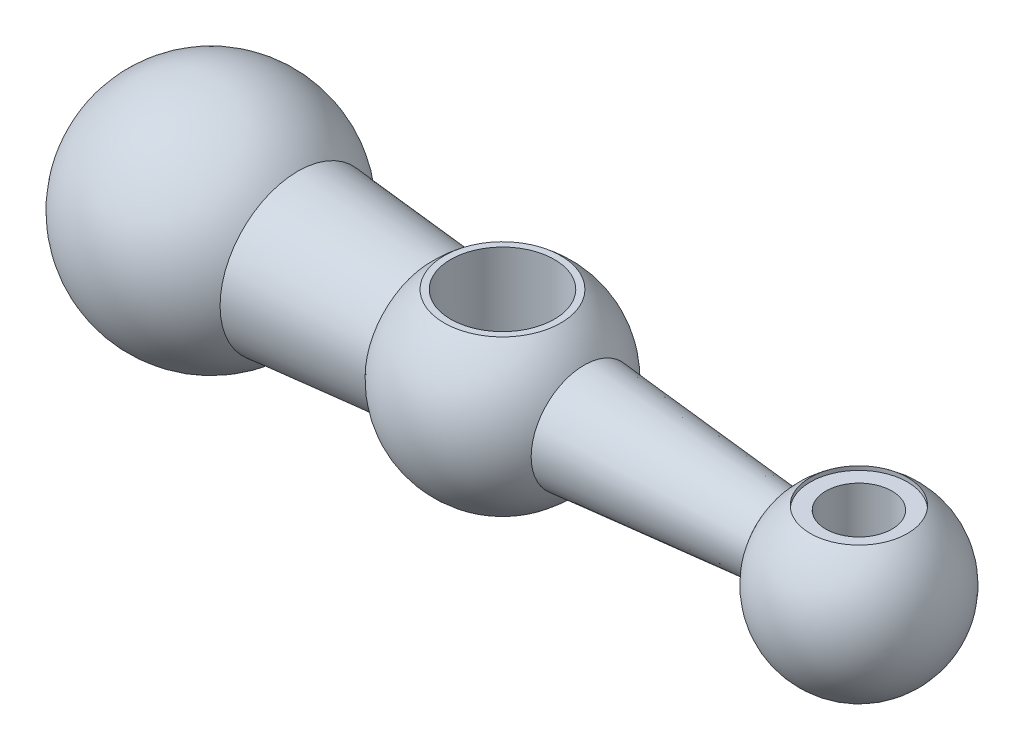
SolidWorks part; units mm, degrees
material "Plain Carbon Steel"
ref_plane "Front Plane" through (0, 0, 0) normal (0, 0, 1) x (1, 0, 0)
ref_plane "Top Plane" through (0, 0, 0) normal (0, 1, 0) x (1, 0, 0)
ref_plane "Right Plane" through (0, 0, 0) normal (1, 0, 0) x (0, 0, -1)
sketch "Handle Profile Sketch" plane through (0, 0, 0) normal (0, 0, 1) x (1, 0, 0)
  line L0 (-65.4913, 0) -> (73.3358, 0) construction
  line L1 (-31.5836, 12) -> (-10.9885, 10.2104)
  line L2 (-63, 0) -> (68, 0)
  line L3 (12.5849, 8.162) -> (43.2208, 5.5)
  arc A0 (-31.5836, 12) -> (-63, 0) centre (-45, 0) ccw
  arc A1 (12.5849, 8.162) -> (-10.9885, 10.2104) centre (0, 0) ccw
  arc A4 (68, 0) -> (43.2208, 5.5) centre (55, 0) ccw
  dimension "D1" = 36
  dimension "D2" = 30
  dimension "D3" = 13
  dimension "D4" = 100
  dimension "D5" = 45
  dimension "D6" = 55.4151
  dimension "D8" = 5.5
revolve "Handle Body Revolve" add sketch "Handle Profile Sketch" angle 360 about L0
sketch "Bore Ø13 Sketch" plane through (0, 0, 0) normal (0, 1, 0) x (1, 0, 0)
  circle A0 centre (0, 0) radius 8
  dimension "D1" = 16
extrude "Bore Ø13" cut sketch "Bore Ø13 Sketch" against normal through all both and the other way through all
sketch "Recess Ø15 Sketch" plane through (0, 0, 0) normal (0, 1, 0) x (1, 0, 0)
  circle A0 centre (55, 0) radius 7.5
  dimension "D1" = 15
  dimension "D2" = 55
extrude "Recess Ø15x10" cut sketch "Recess Ø15 Sketch" along normal through all from offset 10
sketch "Counterbore Ø18 Sketch" plane through (0, 0, 0) normal (0, 1, 0) x (1, 0, 0)
  circle A0 centre (0, 0) radius 9
  dimension "D1" = 18
extrude "Counterbore Ø18x12" cut sketch "Counterbore Ø18 Sketch" along normal through all from offset 12
mirror "Counterbore Mirror" about plane through (0, 0, 0) normal (0, 1, 0) of "Counterbore Ø18x12"
sketch "Sketch5" plane through (0, 0, 0) normal (0, 1, 0) x (1, 0, 0)
  circle A0 centre (55, 0) radius 8.5
  dimension "D1" = 17
sketch "Sketch6" plane through (0, 0, 0) normal (0, 1, 0) x (1, 0, 0)
  circle A0 centre (55, 0) radius 5.1
extrude "Handle Shank Bore Ø10.2" cut sketch "Sketch6" against normal through all and the other way through all
